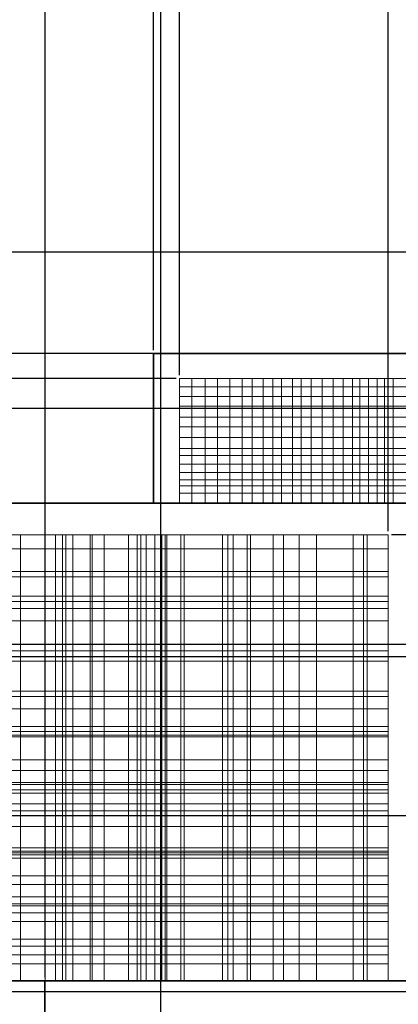
# Model space of a CAD drawing. Units: inches. Extents: x -10 to 130, y -32 to 34.
# Tile 10 of 22: x 42.14 to 49.15, y 5.57 to 23.78. Entities that reach past the tile are written whole.
import ezdxf

# ---------------------------------------------------------------- set-up
doc = ezdxf.new("R2010")
doc.units = ezdxf.units.IN
doc.header["$MEASUREMENT"] = 0
for name, color, linetype, lineweight in [('A-ANNO-DIMS', 2, 'Continuous', 18), ('A-ELEV', 7, 'Continuous', 35), ('A-GLAZ', 4, 'Continuous', 18)]:
    doc.layers.add(name, color=color, linetype=linetype, lineweight=lineweight)
doc.styles.get("Standard").update_dxf_attribs({"font": 'arial.ttf'})
doc.dimstyles.get("Standard").update_dxf_attribs({"dimtxt": 0.18, "dimasz": 0.18, "dimexe": 0.18, "dimexo": 0.0625, "dimgap": 0.09, "dimtad": 0, "dimtih": 1, "dimtoh": 1, "dimdec": 4, "dimzin": 0, "dimdsep": 46, "dimtxsty": 'Standard', "dimcen": 0.09, "dimadec": 0, "dimazin": 0, "dimtfac": 1, "dimtdec": 4, "dimtofl": 0, "dimtmove": 0, "dimatfit": 3, "dimfxl": 1, "dimtolj": 1, "dimtzin": 0, "dimarcsym": 0})

# ---------------------------------------------------------------- blocks, each defined once
blk = doc.blocks.new('*D6')
at = {"layer": 'A-ANNO-DIMS', "color": 0, "lineweight": -2, "transparency": 16777216}
for p, q in [((31.971, 6.07), (31.971, 33.879)), ((42.614, 6.07), (42.614, 33.879)), ((32.151, 33.699), (36.837, 33.699)), ((42.434, 33.699), (37.748, 33.699))]:
    blk.add_line(p, q, dxfattribs=at)
at = {"layer": 'A-ANNO-DIMS', "color": 0, "transparency": 16777216}
for points in [[(32.151, 33.729), (32.151, 33.669), (31.971, 33.699)], [(42.434, 33.729), (42.434, 33.669), (42.614, 33.699)]]:
    blk.add_solid(points, dxfattribs=at)
at = {"layer": 'Defpoints', "color": 0, "transparency": 16777216}
for p in [(42.614, 33.699), (31.971, 6.007), (42.614, 6.007)]:
    blk.add_point(p, dxfattribs=at)
at = {"layer": 'A-ANNO-DIMS', "color": 0, "transparency": 16777216, "insert": (37.293, 33.699), "char_height": 0.18, "attachment_point": 5}
blk.add_mtext('\\A1;10.643', dxfattribs=at)
blk = doc.blocks.new('*D7')
at = {"layer": 'A-ANNO-DIMS', "color": 0, "lineweight": -2, "transparency": 16777216}
for p, q in [((42.614, 6.07), (42.614, 33.879)), ((49.946, 6.07), (49.946, 33.879)), ((42.794, 33.699), (45.888, 33.699)), ((49.766, 33.699), (46.672, 33.699))]:
    blk.add_line(p, q, dxfattribs=at)
at = {"layer": 'A-ANNO-DIMS', "color": 0, "transparency": 16777216}
for points in [[(42.794, 33.729), (42.794, 33.669), (42.614, 33.699)], [(49.766, 33.729), (49.766, 33.669), (49.946, 33.699)]]:
    blk.add_solid(points, dxfattribs=at)
at = {"layer": 'Defpoints', "color": 0, "transparency": 16777216}
for p in [(49.946, 33.699), (42.614, 6.007), (49.946, 6.007)]:
    blk.add_point(p, dxfattribs=at)
at = {"layer": 'A-ANNO-DIMS', "color": 0, "transparency": 16777216, "insert": (46.28, 33.699), "char_height": 0.18, "attachment_point": 5}
blk.add_mtext('\\A1;7.332', dxfattribs=at)
blk = doc.blocks.new('*D17')
at = {"layer": 'A-ANNO-DIMS', "color": 0, "lineweight": -2, "transparency": 16777216}
for p, q in [((39.364, 19.52), (39.364, 33.879)), ((44.622, 17.67), (44.622, 33.879)), ((39.544, 33.699), (41.599, 33.699)), ((44.442, 33.699), (42.387, 33.699))]:
    blk.add_line(p, q, dxfattribs=at)
at = {"layer": 'A-ANNO-DIMS', "color": 0, "transparency": 16777216}
for points in [[(39.544, 33.729), (39.544, 33.669), (39.364, 33.699)], [(44.442, 33.729), (44.442, 33.669), (44.622, 33.699)]]:
    blk.add_solid(points, dxfattribs=at)
at = {"layer": 'Defpoints', "color": 0, "transparency": 16777216}
for p in [(44.622, 33.699), (39.364, 19.458), (44.622, 17.607)]:
    blk.add_point(p, dxfattribs=at)
at = {"layer": 'A-ANNO-DIMS', "color": 0, "transparency": 16777216, "insert": (41.993, 33.699), "char_height": 0.18, "attachment_point": 5}
blk.add_mtext('\\A1;5.257', dxfattribs=at)
blk = doc.blocks.new('*D18')
at = {"layer": 'A-ANNO-DIMS', "color": 0, "lineweight": -2, "transparency": 16777216}
for p, q in [((44.622, 17.67), (44.622, 33.879)), ((50.035, 27.261), (50.035, 33.879)), ((44.802, 33.699), (46.935, 33.699)), ((49.855, 33.699), (47.722, 33.699))]:
    blk.add_line(p, q, dxfattribs=at)
at = {"layer": 'A-ANNO-DIMS', "color": 0, "transparency": 16777216}
for points in [[(44.802, 33.729), (44.802, 33.669), (44.622, 33.699)], [(49.855, 33.729), (49.855, 33.669), (50.035, 33.699)]]:
    blk.add_solid(points, dxfattribs=at)
at = {"layer": 'Defpoints', "color": 0, "transparency": 16777216}
for p in [(50.035, 33.699), (50.035, 27.199), (44.622, 17.607)]:
    blk.add_point(p, dxfattribs=at)
at = {"layer": 'A-ANNO-DIMS', "color": 0, "transparency": 16777216, "insert": (47.328, 33.699), "char_height": 0.18, "attachment_point": 5}
blk.add_mtext('\\A1;5.413', dxfattribs=at)
blk = doc.blocks.new('*D28')
at = {"layer": 'A-ANNO-DIMS', "color": 0, "lineweight": -2, "transparency": 16777216}
for p, q in [((21.715, 14.903), (21.715, 33.879)), ((49.946, 14.903), (49.946, 33.879)), ((21.895, 33.699), (35.436, 33.699)), ((49.766, 33.699), (36.226, 33.699))]:
    blk.add_line(p, q, dxfattribs=at)
at = {"layer": 'A-ANNO-DIMS', "color": 0, "transparency": 16777216}
for points in [[(21.895, 33.729), (21.895, 33.669), (21.715, 33.699)], [(49.766, 33.729), (49.766, 33.669), (49.946, 33.699)]]:
    blk.add_solid(points, dxfattribs=at)
at = {"layer": 'Defpoints', "color": 0, "transparency": 16777216}
for p in [(49.946, 33.699), (21.715, 14.841), (49.946, 14.841)]:
    blk.add_point(p, dxfattribs=at)
at = {"layer": 'A-ANNO-DIMS', "color": 0, "transparency": 16777216, "insert": (35.831, 33.699), "char_height": 0.18, "attachment_point": 5}
blk.add_mtext('\\A1;28.23', dxfattribs=at)
blk = doc.blocks.new('*D34')
at = {"layer": 'A-ANNO-DIMS', "color": 0, "lineweight": -2, "transparency": 16777216}
for p, q in [((13.34, 6.007), (-9.564, 6.007)), ((-9.384, 5.827), (-9.384, 3.941)), ((-9.384, 1.691), (-9.384, 3.577)), ((70.835, 1.511), (-9.564, 1.511))]:
    blk.add_line(p, q, dxfattribs=at)
at = {"layer": 'A-ANNO-DIMS', "color": 0, "transparency": 16777216}
for points in [[(-9.414, 5.827), (-9.354, 5.827), (-9.384, 6.007)], [(-9.414, 1.691), (-9.354, 1.691), (-9.384, 1.511)]]:
    blk.add_solid(points, dxfattribs=at)
at = {"layer": 'Defpoints', "color": 0, "transparency": 16777216}
for p in [(-9.384, 6.007), (13.402, 6.007), (70.898, 1.511)]:
    blk.add_point(p, dxfattribs=at)
at = {"layer": 'A-ANNO-DIMS', "color": 0, "transparency": 16777216, "insert": (-9.384, 3.759), "char_height": 0.18, "attachment_point": 5}
blk.add_mtext('\\A1;4.497', dxfattribs=at)
blk = doc.blocks.new('*D36')
at = {"layer": 'A-ANNO-DIMS', "color": 0, "lineweight": -2, "transparency": 16777216}
for p, q in [((44.559, 17.607), (-9.564, 17.607)), ((-9.384, 17.427), (-9.384, 16.405)), ((-9.384, 15.021), (-9.384, 16.044)), ((21.653, 14.841), (-9.564, 14.841))]:
    blk.add_line(p, q, dxfattribs=at)
at = {"layer": 'A-ANNO-DIMS', "color": 0, "transparency": 16777216}
for points in [[(-9.414, 17.427), (-9.354, 17.427), (-9.384, 17.607)], [(-9.414, 15.021), (-9.354, 15.021), (-9.384, 14.841)]]:
    blk.add_solid(points, dxfattribs=at)
at = {"layer": 'Defpoints', "color": 0, "transparency": 16777216}
for p in [(-9.384, 17.607), (44.622, 17.607), (21.715, 14.841)]:
    blk.add_point(p, dxfattribs=at)
at = {"layer": 'A-ANNO-DIMS', "color": 0, "transparency": 16777216, "insert": (-9.384, 16.224), "char_height": 0.18, "attachment_point": 5}
blk.add_mtext('\\A1;2.77', dxfattribs=at)
blk = doc.blocks.new('*D37')
at = {"layer": 'A-ANNO-DIMS', "color": 0, "lineweight": -2, "transparency": 16777216}
for p, q in [((19.526, 19.485), (-9.564, 19.485)), ((-9.384, 19.305), (-9.384, 18.728)), ((-9.384, 17.787), (-9.384, 18.364)), ((44.559, 17.607), (-9.564, 17.607))]:
    blk.add_line(p, q, dxfattribs=at)
at = {"layer": 'A-ANNO-DIMS', "color": 0, "transparency": 16777216}
for points in [[(-9.414, 19.305), (-9.354, 19.305), (-9.384, 19.485)], [(-9.414, 17.787), (-9.354, 17.787), (-9.384, 17.607)]]:
    blk.add_solid(points, dxfattribs=at)
at = {"layer": 'Defpoints', "color": 0, "transparency": 16777216}
for p in [(-9.384, 19.485), (19.588, 19.485), (44.622, 17.607)]:
    blk.add_point(p, dxfattribs=at)
at = {"layer": 'A-ANNO-DIMS', "color": 0, "transparency": 16777216, "insert": (-9.384, 18.546), "char_height": 0.18, "attachment_point": 5}
blk.add_mtext('\\A1;1.877', dxfattribs=at)
blk = doc.blocks.new('*D48')
at = {"layer": 'A-ANNO-DIMS', "color": 0, "lineweight": -2, "transparency": 16777216}
for p, q in [((44.76, -13.293), (44.76, 33.879)), ((74.492, -13.293), (74.492, 33.879)), ((44.94, 33.699), (59.231, 33.699)), ((74.312, 33.699), (60.021, 33.699))]:
    blk.add_line(p, q, dxfattribs=at)
at = {"layer": 'A-ANNO-DIMS', "color": 0, "transparency": 16777216}
for points in [[(44.94, 33.729), (44.94, 33.669), (44.76, 33.699)], [(74.312, 33.729), (74.312, 33.669), (74.492, 33.699)]]:
    blk.add_solid(points, dxfattribs=at)
at = {"layer": 'Defpoints', "color": 0, "transparency": 16777216}
for p in [(74.492, 33.699), (44.76, -13.356), (74.492, -13.356)]:
    blk.add_point(p, dxfattribs=at)
at = {"layer": 'A-ANNO-DIMS', "color": 0, "transparency": 16777216, "insert": (59.626, 33.699), "char_height": 0.18, "attachment_point": 5}
blk.add_mtext('\\A1;29.73', dxfattribs=at)
blk = doc.blocks.new('*D74')
at = {"layer": 'A-ANNO-DIMS', "color": 0, "lineweight": -2, "transparency": 16777216}
for p, q in [((54.085, 17.607), (-9.564, 17.607)), ((-9.384, 17.427), (-9.384, 17.281)), ((-9.384, 16.771), (-9.384, 16.917)), ((55.856, 16.591), (-9.564, 16.591))]:
    blk.add_line(p, q, dxfattribs=at)
at = {"layer": 'A-ANNO-DIMS', "color": 0, "transparency": 16777216}
for points in [[(-9.414, 17.427), (-9.354, 17.427), (-9.384, 17.607)], [(-9.414, 16.771), (-9.354, 16.771), (-9.384, 16.591)]]:
    blk.add_solid(points, dxfattribs=at)
at = {"layer": 'Defpoints', "color": 0, "transparency": 16777216}
for p in [(54.147, 17.607), (-9.384, 16.591), (55.918, 16.591)]:
    blk.add_point(p, dxfattribs=at)
at = {"layer": 'A-ANNO-DIMS', "color": 0, "transparency": 16777216, "insert": (-9.384, 17.099), "char_height": 0.18, "attachment_point": 5}
blk.add_mtext('\\A1;1.02', dxfattribs=at)
blk = doc.blocks.new('*D82')
at = {"layer": 'A-ANNO-DIMS', "color": 0, "lineweight": -2, "transparency": 16777216}
for p, q in [((19.651, 19.485), (129.508, 19.485)), ((129.328, 19.305), (129.328, 18.728)), ((129.328, 17.787), (129.328, 18.364)), ((68.738, 17.607), (129.508, 17.607))]:
    blk.add_line(p, q, dxfattribs=at)
at = {"layer": 'A-ANNO-DIMS', "color": 0, "transparency": 16777216}
for points in [[(129.298, 19.305), (129.358, 19.305), (129.328, 19.485)], [(129.298, 17.787), (129.358, 17.787), (129.328, 17.607)]]:
    blk.add_solid(points, dxfattribs=at)
at = {"layer": 'Defpoints', "color": 0, "transparency": 16777216}
for p in [(19.588, 19.485), (68.676, 17.607), (129.328, 17.607)]:
    blk.add_point(p, dxfattribs=at)
at = {"layer": 'A-ANNO-DIMS', "color": 0, "transparency": 16777216, "insert": (129.328, 18.546), "char_height": 0.18, "attachment_point": 5}
blk.add_mtext('\\A1;1.877', dxfattribs=at)
blk = doc.blocks.new('*D87')
at = {"layer": 'A-ANNO-DIMS', "color": 0, "lineweight": -2, "transparency": 16777216}
for p, q in [((49.884, 14.841), (-9.564, 14.841)), ((-9.384, 14.661), (-9.384, 13.713)), ((-9.384, 12.402), (-9.384, 13.35)), ((49.884, 12.222), (-9.564, 12.222))]:
    blk.add_line(p, q, dxfattribs=at)
at = {"layer": 'A-ANNO-DIMS', "color": 0, "transparency": 16777216}
for points in [[(-9.414, 14.661), (-9.354, 14.661), (-9.384, 14.841)], [(-9.414, 12.402), (-9.354, 12.402), (-9.384, 12.222)]]:
    blk.add_solid(points, dxfattribs=at)
at = {"layer": 'Defpoints', "color": 0, "transparency": 16777216}
for p in [(49.946, 14.841), (-9.384, 12.222), (49.946, 12.222)]:
    blk.add_point(p, dxfattribs=at)
at = {"layer": 'A-ANNO-DIMS', "color": 0, "transparency": 16777216, "insert": (-9.384, 13.532), "char_height": 0.18, "attachment_point": 5}
blk.add_mtext('\\A1;2.619', dxfattribs=at)
blk = doc.blocks.new('*D88')
at = {"layer": 'A-ANNO-DIMS', "color": 0, "lineweight": -2, "transparency": 16777216}
for p, q in [((49.884, 12.222), (-9.564, 12.222)), ((-9.384, 12.042), (-9.384, 10.822)), ((-9.384, 9.238), (-9.384, 10.458)), ((49.884, 9.058), (-9.564, 9.058))]:
    blk.add_line(p, q, dxfattribs=at)
at = {"layer": 'A-ANNO-DIMS', "color": 0, "transparency": 16777216}
for points in [[(-9.414, 12.042), (-9.354, 12.042), (-9.384, 12.222)], [(-9.414, 9.238), (-9.354, 9.238), (-9.384, 9.058)]]:
    blk.add_solid(points, dxfattribs=at)
at = {"layer": 'Defpoints', "color": 0, "transparency": 16777216}
for p in [(49.946, 12.222), (-9.384, 9.058), (49.946, 9.058)]:
    blk.add_point(p, dxfattribs=at)
at = {"layer": 'A-ANNO-DIMS', "color": 0, "transparency": 16777216, "insert": (-9.384, 10.64), "char_height": 0.18, "attachment_point": 5}
blk.add_mtext('\\A1;3.164', dxfattribs=at)
blk = doc.blocks.new('*D89')
at = {"layer": 'A-ANNO-DIMS', "color": 0, "lineweight": -2, "transparency": 16777216}
for p, q in [((49.884, 9.058), (-9.564, 9.058)), ((-9.384, 8.878), (-9.384, 7.612)), ((-9.384, 5.982), (-9.384, 7.248)), ((49.884, 5.802), (-9.564, 5.802))]:
    blk.add_line(p, q, dxfattribs=at)
at = {"layer": 'A-ANNO-DIMS', "color": 0, "transparency": 16777216}
for points in [[(-9.414, 8.878), (-9.354, 8.878), (-9.384, 9.058)], [(-9.414, 5.982), (-9.354, 5.982), (-9.384, 5.802)]]:
    blk.add_solid(points, dxfattribs=at)
at = {"layer": 'Defpoints', "color": 0, "transparency": 16777216}
for p in [(49.946, 9.058), (-9.384, 5.802), (49.946, 5.802)]:
    blk.add_point(p, dxfattribs=at)
at = {"layer": 'A-ANNO-DIMS', "color": 0, "transparency": 16777216, "insert": (-9.384, 7.43), "char_height": 0.18, "attachment_point": 5}
blk.add_mtext('\\A1;3.256', dxfattribs=at)
blk = doc.blocks.new('*D90')
at = {"layer": 'A-ANNO-DIMS', "color": 0, "lineweight": -2, "transparency": 16777216}
for p, q in [((49.884, 5.802), (-9.564, 5.802)), ((-9.384, 5.622), (-9.384, 4.421)), ((-9.384, 2.855), (-9.384, 4.057)), ((49.884, 2.675), (-9.564, 2.675))]:
    blk.add_line(p, q, dxfattribs=at)
at = {"layer": 'A-ANNO-DIMS', "color": 0, "transparency": 16777216}
for points in [[(-9.414, 5.622), (-9.354, 5.622), (-9.384, 5.802)], [(-9.414, 2.855), (-9.354, 2.855), (-9.384, 2.675)]]:
    blk.add_solid(points, dxfattribs=at)
at = {"layer": 'Defpoints', "color": 0, "transparency": 16777216}
for p in [(49.946, 5.802), (-9.384, 2.675), (49.946, 2.675)]:
    blk.add_point(p, dxfattribs=at)
at = {"layer": 'A-ANNO-DIMS', "color": 0, "transparency": 16777216, "insert": (-9.384, 4.239), "char_height": 0.18, "attachment_point": 5}
blk.add_mtext('\\A1;3.127', dxfattribs=at)
blk = doc.blocks.new('*D95')
at = {"layer": 'A-ANNO-DIMS', "color": 0, "lineweight": -2, "transparency": 16777216}
for p, q in [((-9.384, 12.402), (-9.384, 12.582)), ((49.884, 12.222), (-9.564, 12.222)), ((49.884, 11.995), (-9.564, 11.995)), ((-9.384, 11.815), (-9.384, 11.635)), ((-9.384, 11.635), (-9.564, 11.635))]:
    blk.add_line(p, q, dxfattribs=at)
at = {"layer": 'A-ANNO-DIMS', "color": 0, "transparency": 16777216}
for points in [[(-9.414, 12.402), (-9.354, 12.402), (-9.384, 12.222)], [(-9.414, 11.815), (-9.354, 11.815), (-9.384, 11.995)]]:
    blk.add_solid(points, dxfattribs=at)
at = {"layer": 'Defpoints', "color": 0, "transparency": 16777216}
for p in [(49.946, 12.222), (-9.384, 11.995), (49.946, 11.995)]:
    blk.add_point(p, dxfattribs=at)
at = {"layer": 'A-ANNO-DIMS', "color": 0, "transparency": 16777216, "insert": (-9.957, 11.635), "char_height": 0.18, "attachment_point": 5}
blk.add_mtext('\\A1;0.227', dxfattribs=at)
blk = doc.blocks.new('*D106')
at = {"layer": 'A-ANNO-DIMS', "color": 0, "lineweight": -2, "transparency": 16777216}
for p, q in [((22.665, 14.318), (22.665, 33.879)), ((48.963, 14.318), (48.963, 33.879)), ((22.845, 33.699), (35.349, 33.699)), ((48.783, 33.699), (36.279, 33.699))]:
    blk.add_line(p, q, dxfattribs=at)
at = {"layer": 'A-ANNO-DIMS', "color": 0, "transparency": 16777216}
for points in [[(22.845, 33.729), (22.845, 33.669), (22.665, 33.699)], [(48.783, 33.729), (48.783, 33.669), (48.963, 33.699)]]:
    blk.add_solid(points, dxfattribs=at)
at = {"layer": 'Defpoints', "color": 0, "transparency": 16777216}
for p in [(48.963, 33.699), (22.665, 14.256), (48.963, 14.256)]:
    blk.add_point(p, dxfattribs=at)
at = {"layer": 'A-ANNO-DIMS', "color": 0, "transparency": 16777216, "insert": (35.814, 33.699), "char_height": 0.18, "attachment_point": 5}
blk.add_mtext('\\A1;26.298', dxfattribs=at)
blk = doc.blocks.new('*D107')
at = {"layer": 'A-ANNO-DIMS', "color": 0, "lineweight": -2, "transparency": 16777216}
for p, q in [((48.963, 14.318), (48.963, 33.879)), ((49.946, 14.903), (49.946, 33.879)), ((48.783, 33.699), (48.603, 33.699)), ((50.126, 33.699), (50.306, 33.699))]:
    blk.add_line(p, q, dxfattribs=at)
at = {"layer": 'A-ANNO-DIMS', "color": 0, "transparency": 16777216}
for points in [[(48.783, 33.729), (48.783, 33.669), (48.963, 33.699)], [(50.126, 33.729), (50.126, 33.669), (49.946, 33.699)]]:
    blk.add_solid(points, dxfattribs=at)
at = {"layer": 'Defpoints', "color": 0, "transparency": 16777216}
for p in [(49.946, 33.699), (49.946, 14.841), (48.963, 14.256)]:
    blk.add_point(p, dxfattribs=at)
at = {"layer": 'A-ANNO-DIMS', "color": 0, "transparency": 16777216, "insert": (49.455, 33.699), "char_height": 0.18, "attachment_point": 5}
blk.add_mtext('\\A1;0.983', dxfattribs=at)
blk = doc.blocks.new('*D108')
at = {"layer": 'A-ANNO-DIMS', "color": 0, "lineweight": -2, "transparency": 16777216}
for p, q in [((129.328, 14.841), (129.328, 15.021)), ((129.328, 15.021), (129.508, 15.021)), ((50.009, 14.841), (129.508, 14.841)), ((129.328, 14.436), (129.328, 14.661)), ((49.025, 14.256), (129.508, 14.256))]:
    blk.add_line(p, q, dxfattribs=at)
at = {"layer": 'A-ANNO-DIMS', "color": 0, "transparency": 16777216}
for points in [[(129.298, 14.661), (129.358, 14.661), (129.328, 14.841)], [(129.298, 14.436), (129.358, 14.436), (129.328, 14.256)]]:
    blk.add_solid(points, dxfattribs=at)
at = {"layer": 'Defpoints', "color": 0, "transparency": 16777216}
for p in [(49.946, 14.841), (129.328, 14.841), (48.963, 14.256)]:
    blk.add_point(p, dxfattribs=at)
at = {"layer": 'A-ANNO-DIMS', "color": 0, "transparency": 16777216, "insert": (129.902, 15.021), "char_height": 0.18, "attachment_point": 5}
blk.add_mtext('\\A1;0.585', dxfattribs=at)
blk = doc.blocks.new('*D109')
at = {"layer": 'A-ANNO-DIMS', "color": 0, "lineweight": -2, "transparency": 16777216}
for p, q in [((44.622, 17.67), (44.622, 33.879)), ((45.103, 17.205), (45.103, 33.879)), ((44.442, 33.699), (44.262, 33.699)), ((45.283, 33.699), (45.463, 33.699))]:
    blk.add_line(p, q, dxfattribs=at)
at = {"layer": 'A-ANNO-DIMS', "color": 0, "transparency": 16777216}
for points in [[(44.442, 33.729), (44.442, 33.669), (44.622, 33.699)], [(45.283, 33.729), (45.283, 33.669), (45.103, 33.699)]]:
    blk.add_solid(points, dxfattribs=at)
at = {"layer": 'Defpoints', "color": 0, "transparency": 16777216}
for p in [(45.103, 33.699), (44.622, 17.607), (45.103, 17.143)]:
    blk.add_point(p, dxfattribs=at)
at = {"layer": 'A-ANNO-DIMS', "color": 0, "transparency": 16777216, "insert": (45.839, 33.699), "char_height": 0.18, "attachment_point": 5}
blk.add_mtext('\\A1;0.481', dxfattribs=at)
blk = doc.blocks.new('*D110')
at = {"layer": 'A-ANNO-DIMS', "color": 0, "lineweight": -2, "transparency": 16777216}
for p, q in [((-9.383551, 17.787359), (-9.383551, 17.967359)), ((44.559228, 17.607359), (-9.563551, 17.607359)), ((45.040057, 17.142679), (-9.563551, 17.142679)), ((-9.383551, 16.962679), (-9.383551, 16.782679))]:
    blk.add_line(p, q, dxfattribs=at)
at = {"layer": 'A-ANNO-DIMS', "color": 0, "transparency": 16777216}
for points in [[(-9.413551, 17.787359), (-9.353551, 17.787359), (-9.383551, 17.607359)], [(-9.413551, 16.962679), (-9.353551, 16.962679), (-9.383551, 17.142679)]]:
    blk.add_solid(points, dxfattribs=at)
at = {"layer": 'Defpoints', "color": 0, "transparency": 16777216}
for p in [(-9.383551, 17.607359), (44.621728, 17.607359), (45.102557, 17.142679)]:
    blk.add_point(p, dxfattribs=at)
at = {"layer": 'A-ANNO-DIMS', "color": 0, "transparency": 16777216, "insert": (-9.383551, 17.375019), "char_height": 0.18, "attachment_point": 5}
blk.add_mtext('\\A1;0.465', dxfattribs=at)

msp = doc.modelspace()

# ---------------------------------------------------------------- linework, layer by layer
at = {"layer": 'A-ELEV'}
for p, q in [((44.6217, 14.8409), (44.6217, 17.6074)), ((44.6217, 17.6074), (54.1471, 17.6074)), ((21.7155, 14.8409), (49.9462, 14.8409)), ((20.3124, 6.0074), (49.9462, 6.0074)), ((42.6089, -0.4138), (42.6089, 6.0074))]:
    msp.add_line(p, q, dxfattribs=at)
at = {"layer": 'A-GLAZ'}
for p, q in [((45.1026, 17.1427), (54.1471, 17.1427)), ((45.1026, 14.8409), (45.1026, 17.1427)), ((45.3302, 14.8409), (45.3302, 17.1427)), ((45.5806, 14.8409), (45.5806, 17.1427)), ((45.8083, 14.8409), (45.8083, 17.1427)), ((46.0359, 14.8409), (46.0359, 17.1427)), ((46.2635, 14.8409), (46.2635, 17.1427)), ((46.4457, 14.8409), (46.4457, 17.1427)), ((46.6505, 14.8409), (46.6505, 17.1427)), ((46.8326, 14.8409), (46.8326, 17.1427)), ((46.992, 14.8409), (46.992, 17.1427)), ((47.1969, 14.8409), (47.1969, 17.1427)), ((47.3562, 14.8409), (47.3562, 17.1427)), ((47.5383, 14.8409), (47.5383, 17.1427)), ((47.7432, 14.8409), (47.7432, 17.1427)), ((47.9481, 14.8409), (47.9481, 17.1427)), ((48.1302, 14.8409), (48.1302, 17.1427)), ((48.3021, 14.8409), (48.3021, 17.1427)), ((48.4397, 14.8409), (48.4397, 17.1427)), ((48.6001, 14.8409), (48.6001, 17.1427)), ((48.7605, 14.8409), (48.7605, 17.1427)), ((48.898, 14.8409), (48.898, 17.1427)), ((49.0585, 14.8409), (49.0585, 17.1427)), ((45.1026, 16.9867), (54.1471, 16.9867)), ((45.1026, 16.8085), (54.1471, 16.8085)), ((45.1026, 16.6303), (54.1471, 16.6303)), ((45.1026, 16.4298), (54.1471, 16.4298)), ((45.1026, 16.2515), (54.1471, 16.2515)), ((45.1026, 16.051), (54.1471, 16.051)), ((45.1026, 15.8505), (54.1471, 15.8505)), ((45.1026, 15.7169), (54.1471, 15.7169)), ((45.1026, 15.5609), (54.1471, 15.5609)), ((45.1026, 15.405), (54.1471, 15.405)), ((45.1026, 15.2713), (54.1471, 15.2713)), ((45.1026, 15.1599), (54.1471, 15.1599)), ((45.1026, 15.0262), (54.1471, 15.0262)), ((22.6649, 14.2556), (48.963, 14.2556)), ((42.1629, 6.0074), (42.1629, 14.2556)), ((42.614, 6.0074), (42.614, 14.2556)), ((42.8074, 6.0074), (42.8074, 14.2556)), ((42.9363, 6.0074), (42.9363, 14.2556)), ((43.0008, 6.0074), (43.0008, 14.2556)), ((43.1297, 6.0074), (43.1297, 14.2556)), ((43.452, 6.0074), (43.452, 14.2556)), ((43.4842, 6.0074), (43.4842, 14.2556)), ((43.7098, 6.0074), (43.7098, 14.2556)), ((44.161, 6.0074), (44.161, 14.2556)), ((44.3221, 6.0074), (44.3221, 14.2556)), ((44.3866, 6.0074), (44.3866, 14.2556)), ((44.4833, 6.0074), (44.4833, 14.2556)), ((44.6444, 6.0074), (44.6444, 14.2556)), ((44.6444, 6.0074), (44.6444, 14.2556)), ((44.7733, 6.0074), (44.7733, 14.2556)), ((44.8378, 6.0074), (44.8378, 14.2556)), ((44.87, 6.0074), (44.87, 14.2556)), ((45.1278, 6.0074), (45.1278, 14.2556)), ((45.1923, 6.0074), (45.1923, 14.2556)), ((45.9013, 6.0074), (45.9013, 14.2556)), ((45.9013, 6.0074), (45.9013, 14.2556)), ((45.998, 6.0074), (45.998, 14.2556)), ((45.998, 6.0074), (45.998, 14.2556)), ((46.0947, 6.0074), (46.0947, 14.2556)), ((46.3525, 6.0074), (46.3525, 14.2556)), ((46.417, 6.0074), (46.417, 14.2556)), ((46.8359, 6.0074), (46.8359, 14.2556)), ((47.0293, 6.0074), (47.0293, 14.2556)), ((47.3194, 6.0074), (47.3194, 14.2556)), ((47.6416, 6.0074), (47.6416, 14.2556)), ((48.3184, 6.0074), (48.3184, 14.2556)), ((48.5118, 6.0074), (48.5118, 14.2556)), ((48.5762, 6.0074), (48.5762, 14.2556)), ((48.963, 6.0074), (48.963, 14.2556)), ((22.6649, 13.9954), (48.963, 13.9954)), ((22.6649, 13.5727), (48.963, 13.5727)), ((22.6649, 13.4751), (48.963, 13.4751)), ((22.6649, 13.1174), (48.963, 13.1174)), ((22.6649, 13.0199), (48.963, 13.0199)), ((22.6649, 12.8898), (48.963, 12.8898)), ((22.6649, 12.8898), (48.963, 12.8898)), ((22.6649, 12.6622), (48.963, 12.6622)), ((22.6649, 12.1093), (48.963, 12.1093)), ((22.6649, 11.9142), (48.963, 11.9142)), ((22.6649, 11.3614), (48.963, 11.3614)), ((22.6649, 11.3614), (48.963, 11.3614)), ((22.6649, 11.2638), (48.963, 11.2638)), ((22.6649, 11.0362), (48.963, 11.0362)), ((22.6649, 10.711), (48.963, 10.711)), ((22.6649, 10.711), (48.963, 10.711)), ((22.6649, 10.711), (48.963, 10.711)), ((22.6649, 10.6134), (48.963, 10.6134)), ((22.6649, 10.5484), (48.963, 10.5484)), ((22.6649, 10.5159), (48.963, 10.5159)), ((22.6649, 10.0931), (48.963, 10.0931)), ((22.6649, 9.898), (48.963, 9.898)), ((22.6649, 9.6704), (48.963, 9.6704)), ((22.6649, 9.6379), (48.963, 9.6379)), ((22.6649, 9.5403), (48.963, 9.5403)), ((22.6649, 9.4753), (48.963, 9.4753)), ((22.6649, 9.2802), (48.963, 9.2802)), ((22.6649, 9.1501), (48.963, 9.1501)), ((22.6649, 8.8574), (48.963, 8.8574)), ((22.6649, 8.4672), (48.963, 8.4672)), ((22.6649, 8.4021), (48.963, 8.4021)), ((22.6649, 8.3696), (48.963, 8.3696)), ((22.6649, 8.3371), (48.963, 8.3371)), ((22.6649, 8.2721), (48.963, 8.2721)), ((22.6649, 7.9469), (48.963, 7.9469)), ((22.6649, 7.7843), (48.963, 7.7843)), ((22.6649, 7.5566), (48.963, 7.5566)), ((22.6649, 7.4266), (48.963, 7.4266)), ((22.6649, 7.3941), (48.963, 7.3941)), ((22.6649, 7.264), (48.963, 7.264)), ((22.6649, 7.1014), (48.963, 7.1014)), ((22.6649, 6.7762), (48.963, 6.7762)), ((22.6649, 6.6461), (48.963, 6.6461)), ((22.6649, 6.4835), (48.963, 6.4835)), ((22.6649, 6.3209), (48.963, 6.3209))]:
    msp.add_line(p, q, dxfattribs=at)

# ---------------------------------------------------------------- dimensions: what is measured, and where the dimension line sits
at = {"layer": 'A-ANNO-DIMS'}
for base, p1, p2, override, picture, middle in [((49.9462, 33.6987), (21.7155, 14.8409), (49.9462, 14.8409), {"dimdec": 2, "dimlfac": 1, "dimrnd": 0, "dimzin": 0, "dimdsep": 46, "dimlunit": 2}, '*D28', (35.8308, 33.6987)), ((48.963, 33.6987), (22.6649, 14.2556), (48.963, 14.2556), {"dimdec": 3, "dimlfac": 1, "dimrnd": 0, "dimzin": 0, "dimdsep": 46, "dimlunit": 2}, '*D106', (35.8139, 33.6987)), ((42.614, 33.6987), (31.9712, 6.0074), (42.614, 6.0074), {"dimdec": 3, "dimlfac": 1, "dimrnd": 0, "dimzin": 0, "dimdsep": 46, "dimlunit": 2}, '*D6', (37.2926, 33.6987)), ((44.6217, 33.6987), (39.3644, 19.4575), (44.6217, 17.6074), {"dimdec": 3, "dimlfac": 1, "dimrnd": 0, "dimzin": 0, "dimdsep": 46, "dimlunit": 2}, '*D17', (41.9931, 33.6987)), ((49.9462, 33.6987), (42.614, 6.0074), (49.9462, 6.0074), {"dimdec": 3, "dimlfac": 1, "dimrnd": 0, "dimzin": 0, "dimdsep": 46, "dimlunit": 2}, '*D7', (46.2801, 33.6987)), ((45.1026, 33.6987), (44.6217, 17.6074), (45.1026, 17.1427), {"dimdec": 3, "dimlfac": 1, "dimrnd": 0, "dimzin": 0, "dimdsep": 46, "dimlunit": 2}, '*D109', (45.8389, 33.6987)), ((50.0347, 33.6987), (44.6217, 17.6074), (50.0347, 27.1987), {"dimdec": 3, "dimlfac": 1, "dimrnd": 0, "dimzin": 0, "dimdsep": 46, "dimlunit": 2}, '*D18', (47.3282, 33.6987)), ((74.492, 33.6987), (44.76, -13.3558), (74.492, -13.3558), {"dimdec": 2, "dimlfac": 1, "dimrnd": 0, "dimzin": 0, "dimdsep": 46, "dimlunit": 2}, '*D48', (59.626, 33.6987)), ((49.9462, 33.6987), (48.963, 14.2556), (49.9462, 14.8409), {"dimdec": 3, "dimlfac": 1, "dimrnd": 0, "dimzin": 0, "dimdsep": 46, "dimlunit": 2}, '*D107', (49.4546, 33.6987))]:
    dim = msp.add_linear_dim(base=base, p1=p1, p2=p2, dimstyle='Standard', override=override, dxfattribs=at)
    dim.commit()
    dim.dimension.update_dxf_attribs({"geometry": picture, "text_midpoint": middle})
for base, p1, p2, override, picture, middle in [((-9.3836, 19.4845), (44.6217, 17.6074), (19.5881, 19.4845), {"dimdec": 3, "dimlfac": 1, "dimrnd": 0, "dimzin": 0, "dimdsep": 46, "dimlunit": 2}, '*D37', (-9.3836, 18.5459)), ((129.3277, 17.6074), (19.5881, 19.4845), (68.6759, 17.6074), {"dimdec": 3, "dimlfac": 1, "dimrnd": 0, "dimzin": 0, "dimdsep": 46, "dimlunit": 2}, '*D82', (129.3277, 18.5459)), ((-9.3836, 17.6074), (45.1026, 17.1427), (44.6217, 17.6074), {"dimdec": 3, "dimlfac": 1, "dimrnd": 0, "dimzin": 0, "dimdsep": 46, "dimlunit": 2}, '*D110', (-9.3836, 17.375)), ((-9.3836, 17.6074), (21.7155, 14.8409), (44.6217, 17.6074), {"dimdec": 2, "dimlfac": 1, "dimrnd": 0, "dimzin": 0, "dimdsep": 46, "dimlunit": 2}, '*D36', (-9.3836, 16.2241)), ((-9.3836, 16.5911), (54.1471, 17.6074), (55.9182, 16.5911), {"dimdec": 2, "dimlfac": 1, "dimrnd": 0, "dimzin": 0, "dimdsep": 46, "dimlunit": 2}, '*D74', (-9.3836, 17.0992)), ((129.3277, 14.8409), (48.963, 14.2556), (49.9462, 14.8409), {"dimdec": 3, "dimlfac": 1, "dimrnd": 0, "dimzin": 0, "dimdsep": 46, "dimlunit": 2}, '*D108', (129.9021, 15.0209)), ((-9.3836, 12.2222), (49.9462, 14.8409), (49.9462, 12.2222), {"dimdec": 3, "dimlfac": 1, "dimrnd": 0, "dimzin": 0, "dimdsep": 46, "dimlunit": 2}, '*D87', (-9.3836, 13.5316)), ((-9.3836, 11.9951), (49.9462, 12.2222), (49.9462, 11.9951), {"dimdec": 3, "dimlfac": 1, "dimrnd": 0, "dimzin": 0, "dimdsep": 46, "dimlunit": 2}, '*D95', (-9.9573, 11.6351)), ((-9.3836, 9.058), (49.9462, 12.2222), (49.9462, 9.058), {"dimdec": 3, "dimlfac": 1, "dimrnd": 0, "dimzin": 0, "dimdsep": 46, "dimlunit": 2}, '*D88', (-9.3836, 10.6401)), ((-9.3836, 5.8024), (49.9462, 9.058), (49.9462, 5.8024), {"dimdec": 3, "dimlfac": 1, "dimrnd": 0, "dimzin": 0, "dimdsep": 46, "dimlunit": 2}, '*D89', (-9.3836, 7.4302)), ((-9.3836, 6.0074), (70.898, 1.5107), (13.4021, 6.0074), {"dimdec": 3, "dimlfac": 1, "dimrnd": 0, "dimzin": 0, "dimdsep": 46, "dimlunit": 2}, '*D34', (-9.3836, 3.7591)), ((-9.3836, 2.6753), (49.9462, 5.8024), (49.9462, 2.6753), {"dimdec": 3, "dimlfac": 1, "dimrnd": 0, "dimzin": 0, "dimdsep": 46, "dimlunit": 2}, '*D90', (-9.3836, 4.2388))]:
    dim = msp.add_linear_dim(base=base, p1=p1, p2=p2, angle=90, dimstyle='Standard', override=override, dxfattribs=at)
    dim.commit()
    dim.dimension.update_dxf_attribs({"geometry": picture, "text_midpoint": middle})

doc.saveas('drawing.dxf')
